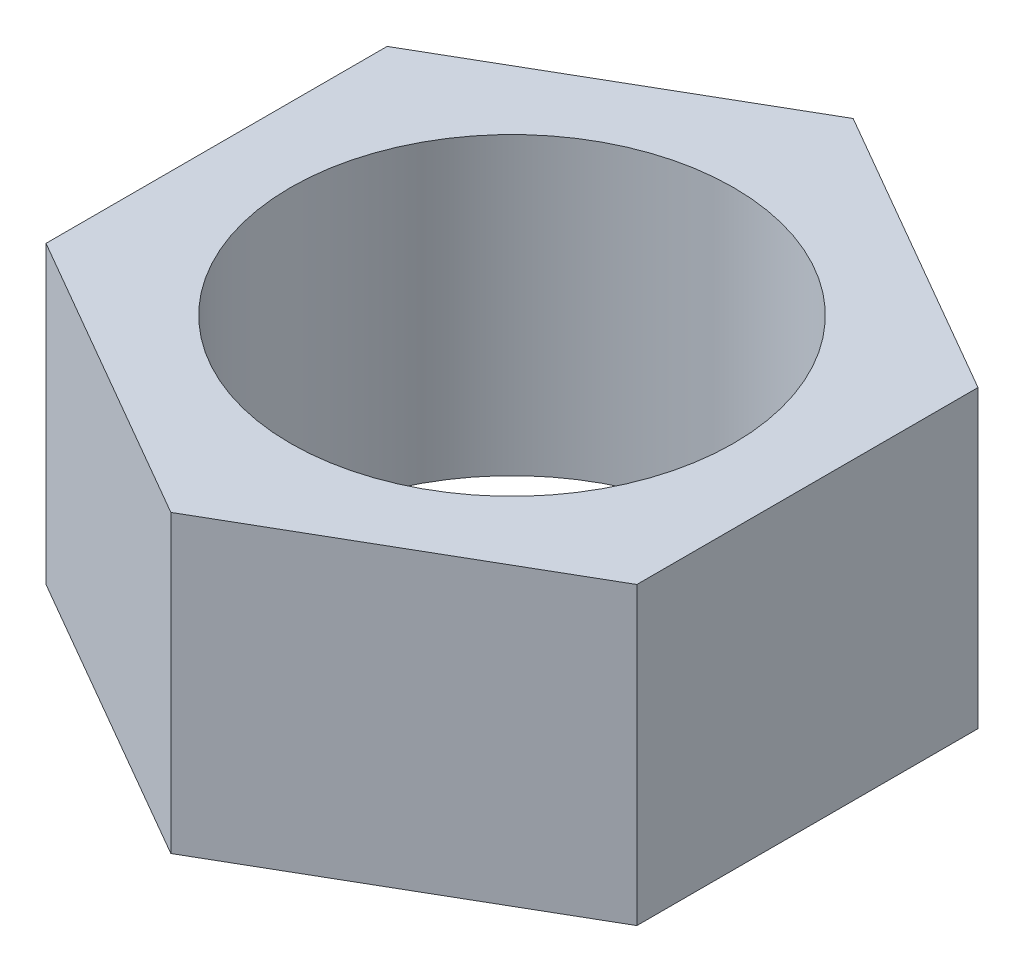
from build123d import *

# Parameters (mm, degrees)
HEX_PROFILE_16AF_WITH_BORE_12_R = 6
NUT_BODY_8_MM_DEPTH             = 4


with BuildPart() as part:
    # Hex Profile 16AF with Bore Ø12 → Nut Body 8 mm (new, symmetric)
    with BuildSketch(Plane(origin=(0, 0, 0), x_dir=(1, 0, 0), z_dir=(0, 1, 0))):
        Polygon((0, -9.237604307), (8, -4.618802154), (8, 4.618802154), (0, 9.237604307), (-8, 4.618802154), (-8, -4.618802154), align=None)
        with Locations(Location((0, 0, 0), (0, 0, 270))):
            Circle(HEX_PROFILE_16AF_WITH_BORE_12_R, mode=Mode.SUBTRACT)
    extrude(amount=NUT_BODY_8_MM_DEPTH, both=True)


solid = part.part
